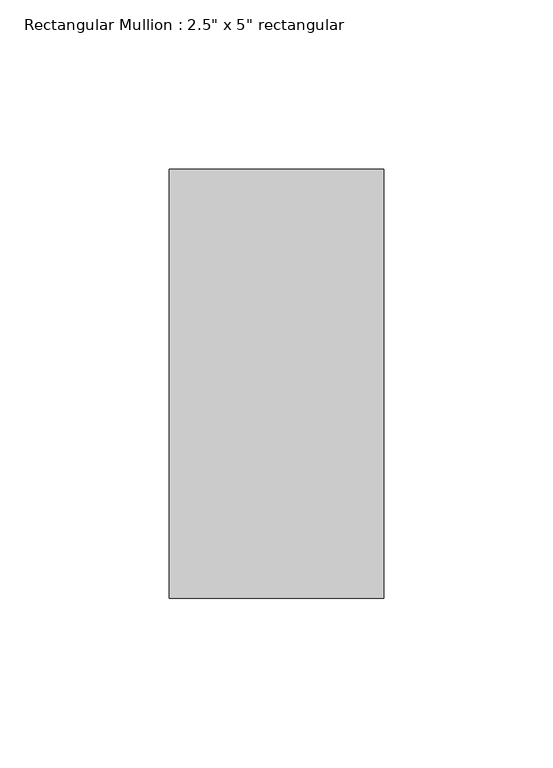
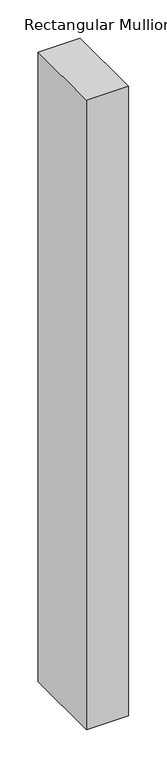
"""IFC4 building model written with IfcOpenShell, lengths in millimetres: member geometry."""

from ifc_helpers import new_model, si_unit, frame, origin, place, context, project, spatial, polyline, outline, extrude, source, transform, mapped, element, save


def member_9a1a11af(model_context):
    return source(origin(), model_context, "Body", "SweptSolid", [
        extrude(outline(polyline([(0.0, 63.5), (0.0, -63.5), (-63.5, -63.5), (-63.5, 63.5), (0.0, 63.5)])), frame((0.0, 0.0, -1004.616916), z_axis=(0.0, 0.0, 1.0), x_axis=(1.0, 0.0, 0.0)), (0.0, 0.0, 1.0), 1004.616916),
    ])


if __name__ == "__main__":
    model = new_model("IFC4")
    model_context = context("Model", 3, world=origin())
    ifc_project = project(units=[si_unit("LENGTHUNIT", "METRE", prefix="MILLI")], contexts=[model_context])
    site = spatial("IfcSite", under=ifc_project)
    building = spatial("IfcBuilding", under=site)
    placement = place(None, origin())
    member_shape = member_9a1a11af(model_context)
    element("IfcMember", 1, ObjectType="Rectangular Mullion : 2.5\" x 5\" rectangular", at=placement, inside=building, context=model_context, shape_type="MappedRepresentation", body=[
        mapped(member_shape, transform((0.0, 0.0, 0.0), x_axis=(1.0, 0.0, 0.0), y_axis=(0.0, 1.0, 0.0), z_axis=(0.0, 0.0, 1.0))),
    ])
    save(model, "model.ifc")

# Revit data of these elements
# Type "Rectangular Mullion : 2.5\" x 5\" rectangular"
#   built-in parameter 1007304 = 0.416667 (stored number, unit not read)
#   built-in parameter 1007301 = 0.104167 (stored number, unit not read)
#   built-in parameter 1007300 = 0.104167 (stored number, unit not read)
# Element 1 (IfcMember, "Rectangular Mullion : 2.5\" x 5\" rectangular")
#   Materials on its faces: "Aluminum"
# Materials
#   "Aluminum": class "Metal", colour RGB 247 247 247, transparency 0, Description = "Aluminum 6061", Cost = 0
